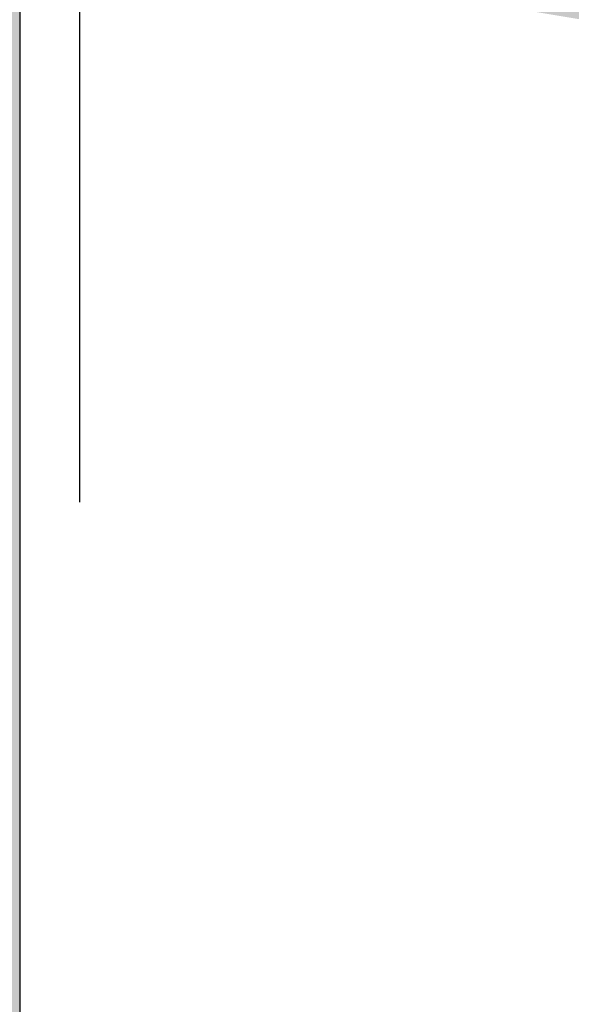
# Model space of a CAD drawing. Units: inches. Extents: x 2091 to 2899, y 967 to 2217.
# Tile 247 of 256: x 2212.144 to 2213.361, y 1137.765 to 1139.939. Entities that reach past the tile are written whole.
import ezdxf

# ---------------------------------------------------------------- set-up
doc = ezdxf.new("R2010")
doc.units = ezdxf.units.IN
doc.layers.add('A-ANNO-DIMS', color=2, linetype='Continuous', lineweight=18)
doc.layers.add('A-WALL-PATT', color=141, linetype='Continuous', lineweight=13, true_color=0xadddf7)
doc.styles.get("Standard").update_dxf_attribs({"font": 'arial.ttf'})
doc.dimstyles.new('ISO-25', dxfattribs={"dimtxt": 4, "dimasz": 4, "dimexe": 1.25, "dimexo": 0.625, "dimtad": 1, "dimdec": 0, "dimlunit": 3, "dimtxsty": 'Standard', "dimcen": 2.5, "dimadec": 0, "dimazin": 0, "dimtfac": 1, "dimtdec": 0, "dimtmove": 0, "dimatfit": 3, "dimfxl": 1, "dimarcsym": 0})

# ---------------------------------------------------------------- blocks, each defined once
blk = doc.blocks.new('*D37')
at = {"layer": 'A-ANNO-DIMS', "color": 0, "lineweight": -2, "transparency": 16777216}
for p, q in [((2203.1157, 1151.6221), (2203.1157, 1138.8736)), ((2212.2756, 1151.6221), (2212.2756, 1138.8736)), ((2199.1157, 1140.1236), (2195.1157, 1140.1236)), ((2203.1157, 1140.1236), (2212.2756, 1140.1236)), ((2216.2756, 1140.1236), (2245.9076, 1140.1236))]:
    blk.add_line(p, q, dxfattribs=at)
at = {"layer": 'A-ANNO-DIMS', "color": 0, "transparency": 16777216}
for points in [[(2199.1157, 1140.7902), (2199.1157, 1139.4569), (2203.1157, 1140.1236)], [(2216.2756, 1140.7902), (2216.2756, 1139.4569), (2212.2756, 1140.1236)]]:
    blk.add_solid(points, dxfattribs=at)
at = {"layer": 'Defpoints', "color": 0, "transparency": 16777216}
for p in [(2203.1157, 1152.2471), (2212.2756, 1152.2471), (2212.2756, 1140.1236)]:
    blk.add_point(p, dxfattribs=at)
at = {"layer": 'A-ANNO-DIMS', "color": 0, "transparency": 16777216, "insert": (2233.0916, 1142.7908), "char_height": 4, "attachment_point": 5}
blk.add_mtext('0\'-9" TYP.', dxfattribs=at)
blk = doc.blocks.new('*D71')
at = {"layer": 'A-ANNO-DIMS', "color": 0, "lineweight": -2, "transparency": 16777216}
for p, q in [((2212.1436, 1351.2941), (2212.1436, 969.4643)), ((2452.1436, 1351.2941), (2452.1436, 969.4643)), ((2216.1436, 970.7143), (2448.1436, 970.7143))]:
    blk.add_line(p, q, dxfattribs=at)
at = {"layer": 'A-ANNO-DIMS', "color": 0, "transparency": 16777216}
for points in [[(2216.1436, 971.381), (2216.1436, 970.0476), (2212.1436, 970.7143)], [(2448.1436, 971.381), (2448.1436, 970.0476), (2452.1436, 970.7143)]]:
    blk.add_solid(points, dxfattribs=at)
at = {"layer": 'Defpoints', "color": 0, "transparency": 16777216}
for p in [(2212.1436, 1351.9191), (2452.1436, 1351.9191), (2452.1436, 970.7143)]:
    blk.add_point(p, dxfattribs=at)
at = {"layer": 'A-ANNO-DIMS', "color": 0, "transparency": 16777216, "insert": (2332.1436, 973.3816), "char_height": 4, "attachment_point": 5}
blk.add_mtext('20\'-0"', dxfattribs=at)
blk = doc.blocks.new('*D75')
at = {"layer": 'A-ANNO-DIMS', "color": 0, "lineweight": -2, "transparency": 16777216}
for p, q in [((2212.1436, 1274.7941), (2212.1436, 969.4643)), ((2308.1436, 1274.7941), (2308.1436, 969.4643)), ((2216.1436, 970.7143), (2304.1436, 970.7143))]:
    blk.add_line(p, q, dxfattribs=at)
at = {"layer": 'A-ANNO-DIMS', "color": 0, "transparency": 16777216}
for points in [[(2216.1436, 971.381), (2216.1436, 970.0476), (2212.1436, 970.7143)], [(2304.1436, 971.381), (2304.1436, 970.0476), (2308.1436, 970.7143)]]:
    blk.add_solid(points, dxfattribs=at)
at = {"layer": 'Defpoints', "color": 0, "transparency": 16777216}
for p in [(2212.1436, 1275.4191), (2308.1436, 1275.4191), (2308.1436, 970.7143)]:
    blk.add_point(p, dxfattribs=at)
at = {"layer": 'A-ANNO-DIMS', "color": 0, "transparency": 16777216, "insert": (2260.1436, 973.3816), "char_height": 4, "attachment_point": 5}
blk.add_mtext('8\'-0"', dxfattribs=at)
blk = doc.blocks.new('*D91')
at = {"layer": 'A-ANNO-DIMS', "color": 0, "lineweight": -2, "transparency": 16777216}
for p, q in [((2211.6506, 1152.2471), (2098.3113, 1152.2471)), ((2099.5613, 1103.9191), (2099.5613, 1148.2471)), ((2211.5186, 1099.9191), (2098.3113, 1099.9191))]:
    blk.add_line(p, q, dxfattribs=at)
at = {"layer": 'A-ANNO-DIMS', "color": 0, "transparency": 16777216}
for points in [[(2098.8947, 1148.2471), (2100.228, 1148.2471), (2099.5613, 1152.2471)], [(2098.8947, 1103.9191), (2100.228, 1103.9191), (2099.5613, 1099.9191)]]:
    blk.add_solid(points, dxfattribs=at)
at = {"layer": 'Defpoints', "color": 0, "transparency": 16777216}
for p in [(2099.5613, 1152.2471), (2212.2756, 1152.2471), (2212.1436, 1099.9191)]:
    blk.add_point(p, dxfattribs=at)
at = {"layer": 'A-ANNO-DIMS', "color": 0, "transparency": 16777216, "insert": (2096.8681, 1126.0831), "char_height": 4, "attachment_point": 5, "rotation": 90}
blk.add_mtext('4\'-4 1/2"', dxfattribs=at)

msp = doc.modelspace()

# ---------------------------------------------------------------- hatches: boundary and pattern name
at = {"layer": 'A-WALL-PATT'}
h = msp.add_hatch(color=256, dxfattribs=at)
h.dxf.hatch_style = 1
h.paths.add_polyline_path([(2803.1436, 2050.9191), (2203.1436, 2050.9191), (2203.1436, 1090.9191), (2803.1436, 1090.9191)])
h.paths.add_polyline_path([(2635.7989, 1147.5405), (2674.5241, 1147.5405, 0.376086), (2678.5297, 1152.8802), (2678.5297, 1159.5565, 0.333335), (2674.5243, 1163.5618), (2674.5243, 1163.5619), (2674.5243, 1192.9344), (2635.806, 1192.9344), (2597.0876, 1192.9344), (2597.0876, 1163.5618, 0.333335), (2593.0823, 1159.5565), (2593.0823, 1152.8802, 0.376086), (2597.0879, 1147.5405)], flags=0)
h.paths.add_polyline_path([(2436.0104, 1278.2408, 0.000483), (2435.9526, 1278.215, -0.001328), (2435.9356, 1278.1117, -0.001711), (2436.1164, 1278.0408, 0.002185)], flags=0)
h.paths.add_polyline_path([(2794.1436, 1143.4191), (2794.1436, 1347.4191), (2543.3702, 1347.4191), (2543.3702, 1351.9191), (2794.1436, 1351.9191), (2794.1436, 1392.7136), (2793.9474, 1392.7136), (2793.9474, 1473.5369), (2794.1436, 1473.5369), (2794.1436, 1531.9191), (2650.1436, 1531.9191), (2650.1436, 1536.4191), (2794.1436, 1536.4191), (2794.1436, 1692.4191), (2609.3756, 1692.4191), (2609.3756, 1644.4191), (2604.8756, 1644.4191), (2604.8756, 1744.9191), (2609.3756, 1744.9191), (2609.3756, 1696.9191), (2794.1436, 1696.9191), (2794.1436, 1780.9191), (2609.6436, 1780.9191), (2493.8756, 1780.9191), (2493.8756, 1785.4191), (2609.6436, 1785.4191), (2794.1436, 1785.4191), (2794.1436, 1847.9388), (2793.9512, 1847.9388), (2793.9512, 1928.7622), (2794.1436, 1928.7622), (2794.1436, 1941.4191), (2614.1436, 1941.4191), (2614.1436, 1821.4191), (2609.6436, 1821.4191), (2609.6436, 1941.4191), (2392.1436, 1941.4191), (2392.1436, 1819.9191), (2387.6436, 1819.9191), (2387.6436, 1941.4191), (2212.1436, 1941.4191), (2212.1436, 1783.9191), (2392.1436, 1783.9191), (2392.1436, 1780.9191), (2212.1436, 1780.9191), (2212.1436, 1629.4191), (2387.6436, 1629.4191), (2387.6436, 1744.9191), (2392.1436, 1744.9191), (2392.1436, 1627.9191), (2317.1436, 1627.9191), (2317.1436, 1551.4191), (2317.1436, 1536.4191), (2459.3836, 1536.4191), (2459.3836, 1602.3965), (2463.8836, 1602.3965), (2463.8836, 1531.9191), (2456.6436, 1531.9191), (2456.6436, 1529.9191), (2452.1436, 1529.9191), (2452.1436, 1531.9191), (2312.6436, 1531.9191), (2312.6436, 1551.4191), (2306.1436, 1551.4191), (2306.1436, 1555.9191), (2308.1436, 1555.9191), (2308.1436, 1551.4191), (2312.6436, 1551.4191), (2312.6436, 1627.9191), (2212.1436, 1627.9191), (2212.1436, 1555.9191), (2270.1436, 1555.9191), (2270.1436, 1551.4191), (2212.1436, 1551.4191), (2212.1436, 1351.9191), (2272.1436, 1351.9191), (2272.1436, 1347.4191), (2212.1436, 1347.4191), (2212.1436, 1275.4191), (2308.1436, 1275.4191), (2308.1436, 1351.9191), (2452.1436, 1351.9191), (2452.1436, 1493.9191), (2456.6436, 1493.9191), (2456.6436, 1347.4191), (2312.6436, 1347.4191), (2312.6436, 1270.9191), (2212.1436, 1270.9191), (2212.1436, 1099.9191), (2281.2375, 1099.9191), (2282.871, 1110.9138), (2282.0083, 1116.9966), (2278.5577, 1121.4204), (2268.2056, 1128.0562), (2272.0876, 1128.0562), (2273.8129, 1131.927), (2279.4203, 1134.6919), (2285.0278, 1135.2449), (2287.6158, 1137.4568), (2288.0471, 1138.0098), (2289.3411, 1140.7747), (2291.0665, 1139.6687), (2292.3605, 1135.2449), (2295.3798, 1136.9038), (2296.2425, 1135.7979), (2297.1052, 1133.033), (2300.1246, 1138.0098), (2303.1439, 1138.0098), (2304.4379, 1135.7979), (2303.1439, 1133.586), (2306.5946, 1134.6919), (2307.8887, 1133.033), (2310.908, 1135.2449), (2313.9274, 1134.1389), (2315.6269, 1132.4271), (2308.32, 1117.5496), (2290.2038, 1109.8079), (2288.9098, 1103.1721), (2289.2723, 1099.9191), (2434.9182, 1099.9191), (2431.5932, 1124.7881), (2429.9302, 1169.5531), (2430.9272, 1240.5197), (2435.6589, 1238.1861), (2437.1352, 1196.5541), (2438.7982, 1143.9731), (2442.6782, 1111.9981), (2446.5582, 1099.9191), (2794.1436, 1099.9191), (2794.1436, 1138.9191), (2548.0324, 1138.9191), (2548.0324, 1143.4191), (2548.0324, 1148.8191), (2546.6685, 1148.0316), (2528.6857, 1179.1786, 0.256256), (2512.0324, 1148.8191), (2512.0324, 1143.4191), (2512.0324, 1138.9191), (2507.5324, 1138.9191), (2507.5324, 1143.4191), (2507.5324, 1148.8191, 0.256256), (2490.8792, 1179.1786), (2472.8964, 1148.0316), (2471.5324, 1148.8191), (2471.5324, 1143.4191), (2467.0324, 1143.4191), (2467.0324, 1269.9458, 0.039061), (2460.91, 1273.5801), (2467.0324, 1273.5801), (2467.0324, 1286.3254, 0.014511), (2465.2162, 1286.7619), (2467.0324, 1287.0526), (2467.0324, 1323.4191), (2471.5324, 1323.4191), (2471.5324, 1148.8191), (2489.5324, 1179.996), (2490.8964, 1179.2085), (2490.8792, 1179.1786, -0.256256), (2507.5324, 1148.8191), (2507.5324, 1143.4191), (2512.0324, 1143.4191), (2512.0324, 1148.8191, -0.256256), (2528.6857, 1179.1786), (2528.6685, 1179.2085), (2530.0324, 1179.996), (2548.0324, 1148.8191), (2548.0324, 1143.4191)], flags=16)
h.paths.add_polyline_path([(2607.7685, 1200.9451), (2607.7685, 1265.0306), (2597.0876, 1281.052), (2619.7846, 1281.052), (2627.7953, 1337.1269), (2635.7989, 1337.1269), (2643.8167, 1337.1269), (2651.8274, 1281.052), (2674.5243, 1281.052), (2663.8434, 1265.0306), (2663.8434, 1200.9451), (2635.806, 1200.9451)], flags=0)
edge = h.paths.add_edge_path(flags=0)
edge.add_ellipse((13303.8962, 1272.9987), major_axis=(-10595.313, 0), ratio=0.8423038701, start_angle=0.62823722, end_angle=0.6465541, ccw=False)
edge.add_ellipse((2711.7004, 1156.8527), major_axis=(2.2198, 0), ratio=0.842304, start_angle=111.5352, end_angle=180.6282, ccw=False)
edge.add_ellipse((13303.1563, 1272.9987), major_axis=(-10593.0263, 0), ratio=0.8423038695, start_angle=0.52827147, end_angle=0.6465541, ccw=False)
edge.add_line((2710.7646, 1175.3333), (2710.13, 1175.3333))
edge.add_ellipse((2710.13, 1176.5798), major_axis=(1.4798, 0), ratio=0.842304, start_angle=180, end_angle=270, ccw=False)
edge.add_line((2708.6501, 1176.5798), (2708.6501, 1200.7829))
edge.add_ellipse((2710.13, 1200.7829), major_axis=(1.4798, 0), ratio=0.842304, start_angle=90, end_angle=180, ccw=False)
edge.add_line((2710.13, 1202.0294), (2710.4651, 1202.0294))
edge.add_ellipse((13303.1563, 1272.9987), major_axis=(-10593.0263, 0), ratio=0.8423038695, start_angle=-0.09022909, end_angle=0.38386678, ccw=False)
edge.add_ellipse((2710.13, 1290.927), major_axis=(-1.4798, 0), ratio=0.842304, start_angle=0, end_angle=90, ccw=False)
edge.add_line((2708.6501, 1290.927), (2708.6501, 1315.1302))
edge.add_ellipse((2710.13, 1315.1302), major_axis=(-1.4798, 0), ratio=0.842304, start_angle=-90, end_angle=0, ccw=False)
edge.add_line((2710.13, 1316.3767), (2710.7063, 1316.3767))
edge.add_ellipse((3238.4017, 1296.2896), major_axis=(528.234, 0), ratio=0.84230387, start_angle=176.349572, end_angle=177.82005, ccw=False)
edge.add_ellipse((2775.063, 1071.4507), major_axis=(313.3078, 0), ratio=0.84230387, start_angle=102.125966, end_angle=103.780529, ccw=False)
edge.add_ellipse((2775.063, 1078.3057), major_axis=(-305.3029, 0), ratio=0.84230387, start_angle=-79.790461, end_angle=-77.555373, ccw=False)
edge.add_ellipse((2695.1418, 1541.9754), major_axis=(-250.9602, 0), ratio=0.84230387, start_angle=99.256566, end_angle=102.554933)
edge.add_line((2741.4103, 1334.2143), (2747.1325, 1337.3785))
edge.add_ellipse((2747.5386, 1336.8575), major_axis=(-0.7399, 0), ratio=0.842304, start_angle=270, end_angle=307.9331, ccw=False)
edge.add_ellipse((2747.5386, 1336.8575), major_axis=(-0.7399, 0), ratio=0.842304, start_angle=232.0669, end_angle=270, ccw=False)
edge.add_line((2747.9447, 1337.3785), (2753.6669, 1334.2143))
edge.add_ellipse((2799.9355, 1541.9754), major_axis=(250.9602, 0), ratio=0.84230387, start_angle=257.445067, end_angle=260.743434)
edge.add_ellipse((2720.0142, 1078.3057), major_axis=(305.3029, 0), ratio=0.84230387, start_angle=77.555373, end_angle=79.790461, ccw=False)
edge.add_ellipse((2720.0142, 1071.4507), major_axis=(-313.3078, 0), ratio=0.84230387, start_angle=256.219471, end_angle=257.874034, ccw=False)
edge.add_ellipse((2256.6755, 1296.2896), major_axis=(-528.234, 0), ratio=0.84230387, start_angle=182.17995, end_angle=183.650428, ccw=False)
edge.add_line((2784.3709, 1316.3767), (2784.9472, 1316.3767))
edge.add_ellipse((2784.9472, 1315.1302), major_axis=(1.4798, 0), ratio=0.842304, start_angle=0, end_angle=90, ccw=False)
edge.add_line((2786.4271, 1315.1302), (2786.4271, 1290.927))
edge.add_ellipse((2784.9472, 1290.927), major_axis=(1.4798, 0), ratio=0.842304, start_angle=270, end_angle=360, ccw=False)
edge.add_ellipse((-7808.0791, 1272.9987), major_axis=(10593.0263, 0), ratio=0.8423038695, start_angle=-0.38386678, end_angle=0.09022909, ccw=False)
edge.add_line((2784.6122, 1202.0294), (2784.9472, 1202.0294))
edge.add_ellipse((2784.9472, 1200.7829), major_axis=(1.4798, 0), ratio=0.842304, start_angle=0, end_angle=90, ccw=False)
edge.add_line((2786.4271, 1200.7829), (2786.4271, 1176.5798))
edge.add_ellipse((2784.9472, 1176.5798), major_axis=(-1.4798, 0), ratio=0.842304, start_angle=90, end_angle=180, ccw=False)
edge.add_line((2784.9472, 1175.3333), (2784.3126, 1175.3333))
edge.add_ellipse((-7808.0791, 1272.9987), major_axis=(10593.0263, 0), ratio=0.8423038695, start_angle=-0.6186432, end_angle=-0.52827147, ccw=False)
edge.add_ellipse((2783.3768, 1156.8527), major_axis=(-2.2198, 0), ratio=0.842304, start_angle=179.3718, end_angle=248.4648, ccw=False)
edge.add_ellipse((-7808.819, 1272.9987), major_axis=(-10595.313, 0), ratio=0.8423038658, start_angle=179.35344592, end_angle=179.3717628, ccw=False)
edge.add_ellipse((2780.2973, 1153.5008), major_axis=(-5.2464, 0), ratio=0.842304, start_angle=90, end_angle=179.3534, ccw=False)
edge.add_line((2780.2973, 1149.0817), (2714.7799, 1149.0817))
edge.add_ellipse((2714.7799, 1153.5008), major_axis=(5.2464, 0), ratio=0.842304, start_angle=180.6466, end_angle=270, ccw=False)
edge = h.paths.add_edge_path(flags=0)
edge.add_line((2718.1874, 1151.0078), (2718.1874, 1170.4724))
edge.add_ellipse((2721.1471, 1170.4724), major_axis=(-2.9597, 0), ratio=0.842304, start_angle=-90, end_angle=0, ccw=False)
edge.add_line((2721.1471, 1172.9653), (2773.9302, 1172.9653))
edge.add_ellipse((2773.9302, 1170.4724), major_axis=(-2.9597, 0), ratio=0.842304, start_angle=180, end_angle=270, ccw=False)
edge.add_line((2776.8899, 1170.4724), (2776.8899, 1151.0078))
edge.add_line((2776.8899, 1151.0078), (2718.1874, 1151.0078))
edge = h.paths.add_edge_path(flags=0)
edge.add_line((2718.1874, 1180.2342), (2718.1874, 1199.0578))
edge.add_ellipse((2747.5386, 1320.3986), major_axis=(147.0179, 0), ratio=0.84230387, start_angle=256.401865, end_angle=283.598135)
edge.add_line((2776.8899, 1199.0578), (2776.8899, 1180.2342))
edge.add_ellipse((2747.5386, 1301.575), major_axis=(147.0179, 0), ratio=0.84230387, start_angle=256.401865, end_angle=283.598135, ccw=False)
edge = h.paths.add_edge_path(flags=0)
edge.add_ellipse((13303.1563, 1272.9987), major_axis=(-10591.5465, 0), ratio=0.8423038696, start_angle=0.05559431, end_angle=0.37776419, ccw=False)
edge.add_line((2711.6169, 1262.7217), (2715.6674, 1249.4954))
edge.add_ellipse((6413.892, 1241.6919), major_axis=(-3698.2362, 0), ratio=0.84230387, start_angle=-0.1208974, end_angle=0.3640763)
edge.add_line((2715.761, 1218.1925), (2711.9343, 1203.1674))
edge = h.paths.add_edge_path(flags=0)
edge.add_line((2718.1874, 1251.0746), (2716.0025, 1267.4504))
edge.add_ellipse((2742.1512, 1202.1895), major_axis=(81.7726, 0), ratio=0.8423039, start_angle=94.277421, end_angle=111.834954, ccw=False)
edge.add_line((2737.0097, 1270.9306), (2758.0675, 1270.9306))
edge.add_ellipse((2752.9261, 1202.1895), major_axis=(81.7726, 0), ratio=0.8423039, start_angle=68.165046, end_angle=85.722579, ccw=False)
edge.add_line((2779.0747, 1267.4504), (2776.8899, 1251.0746))
edge.add_ellipse((2750.3381, 1187.8854), major_axis=(79.5797, 0), ratio=0.8423039, start_angle=67.208085, end_angle=85.12993)
edge.add_line((2756.0347, 1254.7437), (2739.0426, 1254.7437))
edge.add_ellipse((2744.7392, 1187.8854), major_axis=(79.5797, 0), ratio=0.8423039, start_angle=94.87007, end_angle=112.791915)
edge = h.paths.add_edge_path(flags=0)
edge.add_line((2783.1429, 1203.1674), (2779.3162, 1218.1925))
edge.add_ellipse((-918.8147, 1241.6919), major_axis=(3698.2362, 0), ratio=0.84230387, start_angle=-0.3640763, end_angle=0.1208974)
edge.add_line((2779.4098, 1249.4954), (2783.4604, 1262.7217))
edge.add_ellipse((-7808.0791, 1272.9987), major_axis=(-10591.5465, 0), ratio=0.8423038695, start_angle=179.62223581, end_angle=179.94440569, ccw=False)
edge = h.paths.add_edge_path(flags=0)
edge.add_ellipse((2734.2009, 1286.6904), major_axis=(-0.3566, 6.3401), ratio=0.603834, start_angle=89.00201, end_angle=253.65741, ccw=False)
edge.add_line((2730.369, 1286.5418), (2730.369, 1301.352))
edge.add_line((2730.369, 1301.352), (2735.9133, 1305.2148))
edge.add_ellipse((2736.3849, 1304.7346), major_axis=(0.7399, 0), ratio=0.842304, start_angle=90, end_angle=134.4802, ccw=False)
edge.add_line((2736.3849, 1305.3578), (2738.0328, 1305.3578))
edge.add_line((2738.0328, 1305.3578), (2738.0328, 1307.7079))
edge.add_ellipse((2794.2016, 1307.7079), major_axis=(56.1689, 0), ratio=0.8423039, start_angle=150.56143, end_angle=180, ccw=False)
edge.add_ellipse((2700.8756, 1307.7079), major_axis=(-56.1689, 0), ratio=0.8423039, start_angle=180, end_angle=209.43857, ccw=False)
edge.add_line((2757.0444, 1307.7079), (2757.0444, 1305.3578))
edge.add_line((2757.0444, 1305.3578), (2758.6923, 1305.3578))
edge.add_ellipse((2758.6923, 1304.7346), major_axis=(-0.7399, 0), ratio=0.842304, start_angle=225.5198, end_angle=270, ccw=False)
edge.add_line((2759.1639, 1305.2148), (2764.7082, 1301.352))
edge.add_line((2764.7082, 1301.352), (2764.7082, 1286.5418))
edge.add_ellipse((2760.8763, 1286.6904), major_axis=(0.3566, 6.3401), ratio=0.603834, start_angle=106.34259, end_angle=270.99799, ccw=False)
edge.add_line((2757.0444, 1285.7971), (2757.0444, 1307.7079))
edge.add_ellipse((2700.8756, 1307.7079), major_axis=(-56.1689, 0), ratio=0.8423039, start_angle=180, end_angle=209.43857)
edge.add_ellipse((2794.2016, 1307.7079), major_axis=(56.1689, 0), ratio=0.8423039, start_angle=150.56143, end_angle=180)
edge.add_line((2738.0328, 1307.7079), (2738.0328, 1285.7971))
h.paths.add_polyline_path([(2417.8123, 1104.4497), (2413.4923, 1102.5297), (2410.6123, 1103.9697), (2409.1723, 1106.3697), (2407.2523, 1107.3297), (2406.2923, 1109.7297), (2405.3323, 1114.0497), (2405.3323, 1117.8897), (2406.2923, 1120.1297), (2407.2523, 1119.8097), (2408.8483, 1118.3277), (2410.1739, 1119.4242), (2410.2113, 1120.4057), (2411.0407, 1121.4191), (2410.6993, 1119.8587), (2410.1739, 1119.4242), (2410.0885, 1117.1761), (2411.1328, 1116.2063), (2413.9723, 1119.3297), (2416.8523, 1120.7697), (2416.8697, 1120.7988), (2417.0351, 1119.4051), (2417.8962, 1118.1434), (2418.2923, 1118.3697), (2419.5444, 1120.0393), (2419.3609, 1118.3875), (2419.0321, 1119.3562), (2418.3989, 1118.5119), (2419.2523, 1114.5297), (2418.7941, 1107.1988)], flags=0)
h.paths.add_polyline_path([(2508.8702, 1347.4191), (2508.3702, 1347.4191), (2508.3702, 1351.9191), (2508.8702, 1351.9191)], flags=0)
h.paths.add_polyline_path([(2473.3702, 1347.4191), (2472.3702, 1347.4191), (2467.8702, 1347.4191), (2467.8702, 1455.4191), (2472.3702, 1455.4191), (2472.3702, 1352.4191), (2473.3702, 1352.4191)], flags=0)
h.paths.add_polyline_path([(2352.1062, 1217.4462), (2349.2262, 1218.8862), (2347.7862, 1221.2862), (2345.8662, 1222.2462), (2344.9062, 1224.6462), (2343.9462, 1228.9662), (2343.9462, 1232.8062), (2344.9062, 1235.0462), (2345.8662, 1234.7262), (2347.4623, 1233.2442), (2348.7879, 1234.3407), (2348.8252, 1235.3222), (2349.6547, 1236.3355), (2349.3132, 1234.7752), (2348.7879, 1234.3407), (2348.7024, 1232.0926), (2349.7468, 1231.1228), (2352.5862, 1234.2462), (2355.4662, 1235.6862), (2355.4837, 1235.7153), (2355.649, 1234.3216), (2356.5102, 1233.0599), (2356.9062, 1233.2862), (2358.1584, 1234.9558), (2357.9749, 1233.304), (2357.6461, 1234.2726), (2357.0129, 1233.4284), (2357.8662, 1229.4462), (2357.4081, 1222.1153), (2356.4262, 1219.3662)], flags=0)
h.paths.add_polyline_path([(2348.2968, 1112.2244), (2347.0138, 1112.3104), (2345.5298, 1114.1274), (2345.7318, 1115.8584), (2346.8118, 1116.9824), (2346.8118, 1114.6464), (2345.8668, 1114.2144), (2346.8798, 1114.3004)], flags=0)
h.paths.add_polyline_path([(2347.0138, 1110.9264), (2346.2718, 1110.4934), (2346.6098, 1111.1864)], flags=0)
h.paths.add_polyline_path([(2345.8668, 1118.1944), (2345.5298, 1117.3294), (2343.7078, 1118.0214), (2344.3828, 1118.6264)], flags=0)
h.paths.add_polyline_path([(2346.6768, 1109.2824), (2346.0698, 1108.0714), (2345.8668, 1110.0614)], flags=0)
h.paths.add_polyline_path([(2345.0568, 1119.7514), (2343.6398, 1119.7514), (2343.9778, 1121.1354)], flags=0)
h.paths.add_polyline_path([(2345.2598, 1116.5504), (2345.1248, 1115.8584), (2344.9218, 1115.6854), (2344.7198, 1116.3774)], flags=0)
h.paths.add_polyline_path([(2345.6648, 1112.3104), (2345.4618, 1111.5324), (2344.0448, 1111.9644), (2344.6518, 1112.5704)], flags=0)
h.paths.add_polyline_path([(2345.1918, 1113.3494), (2344.4498, 1113.8684), (2344.7198, 1114.3874)], flags=0)
h.paths.add_polyline_path([(2344.6518, 1116.8094), (2344.1798, 1115.6854), (2344.6518, 1115.3394), (2343.9098, 1114.9064), (2343.0328, 1115.9444), (2343.6398, 1116.4634)], flags=0)
h.paths.add_polyline_path([(2345.8668, 1106.6864), (2344.9898, 1105.5624), (2344.5168, 1106.6004)], flags=0)
h.paths.add_polyline_path([(2344.8548, 1110.0614), (2344.5168, 1109.2824), (2344.1128, 1109.7154)], flags=0)
h.paths.add_polyline_path([(2344.0448, 1113.5224), (2343.4378, 1113.0894), (2342.7628, 1113.9544)], flags=0)
h.paths.add_polyline_path([(2344.3148, 1111.0124), (2342.9648, 1110.3204), (2342.9648, 1111.0994)], flags=0)
h.paths.add_polyline_path([(2345.1248, 1104.6974), (2344.5848, 1103.7454), (2344.4498, 1104.2644)], flags=0)
h.paths.add_polyline_path([(2342.8298, 1121.2224), (2341.7498, 1120.5304), (2340.5358, 1121.0494), (2340.1308, 1121.8284), (2340.6708, 1122.9524), (2341.1428, 1121.8284), (2341.6148, 1122.0014)], flags=0)
h.paths.add_polyline_path([(2342.9648, 1119.7514), (2343.0328, 1118.4534), (2342.0878, 1118.0214), (2342.0198, 1119.4914)], flags=0)
h.paths.add_polyline_path([(2342.6948, 1116.8964), (2341.9528, 1116.6364), (2342.0198, 1117.3294)], flags=0)
h.paths.add_polyline_path([(2343.0328, 1112.2244), (2342.0198, 1111.7914), (2341.5478, 1112.2244), (2342.3578, 1113.3494)], flags=0)
h.paths.add_polyline_path([(2343.7748, 1104.4374), (2342.6278, 1102.8804), (2342.6948, 1104.6104), (2343.4378, 1105.1294)], flags=0)
h.paths.add_polyline_path([(2342.0198, 1115.0794), (2340.8058, 1115.5124), (2340.9408, 1116.3774)], flags=0)
h.paths.add_polyline_path([(2341.4808, 1120.0974), (2341.4808, 1119.4054), (2341.0758, 1119.5784), (2341.1428, 1120.0974)], flags=0)
h.paths.add_polyline_path([(2341.8178, 1114.4734), (2340.9408, 1113.0894), (2340.8058, 1114.5604)], flags=0)
h.paths.add_polyline_path([(2341.1428, 1118.5404), (2340.9408, 1116.9824), (2339.0508, 1117.6754), (2339.0508, 1118.6264)], flags=0)
h.paths.add_polyline_path([(2342.6948, 1101.6684), (2341.9528, 1101.8414), (2342.5598, 1102.3614)], flags=0)
h.paths.add_polyline_path([(2340.3328, 1119.6654), (2338.4438, 1119.5784), (2337.9038, 1120.3574), (2339.6578, 1120.6164)], flags=0)
h.paths.add_polyline_path([(2340.3328, 1115.3394), (2340.0628, 1113.6954), (2339.3878, 1115.3394)], flags=0)
h.paths.add_polyline_path([(2341.8178, 1103.8314), (2341.5478, 1102.8804), (2341.1428, 1103.6584)], flags=0)
h.paths.add_polyline_path([(2339.0508, 1122.8664), (2337.2958, 1121.8284), (2337.0938, 1123.1254), (2337.7688, 1123.8184)], flags=0)
h.paths.add_polyline_path([(2339.1178, 1121.7414), (2338.8478, 1121.2224), (2338.1738, 1121.0494), (2338.3758, 1121.5684)], flags=0)
h.paths.add_polyline_path([(2339.1858, 1119.3194), (2338.6458, 1118.7134), (2338.2408, 1118.1074), (2338.2408, 1118.8864)], flags=0)
h.paths.add_polyline_path([(2341.1428, 1101.9284), (2340.6028, 1101.2364), (2340.0628, 1101.8414), (2340.6028, 1102.3614)], flags=0)
h.paths.add_polyline_path([(2337.6338, 1117.7614), (2336.6208, 1118.2804), (2337.2958, 1118.9724)], flags=0)
h.paths.add_polyline_path([(2336.8238, 1119.5784), (2334.7988, 1118.9724), (2335.2038, 1120.3574), (2336.5538, 1120.8764)], flags=0)
h.paths.add_polyline_path([(2339.1178, 1100.4574), (2337.3638, 1100.5434), (2336.7558, 1101.2364)], flags=0)
h.paths.add_polyline_path([(2336.3508, 1122.4334), (2336.0138, 1121.9144), (2334.9338, 1122.4334), (2334.5288, 1123.4714), (2335.7438, 1122.7794)], flags=0)
h.paths.add_polyline_path([(2334.7318, 1120.8764), (2334.2588, 1120.3574), (2334.0568, 1120.7894), (2334.5968, 1121.3084)], flags=0)
h.paths.add_polyline_path([(2334.4618, 1122.1744), (2332.5718, 1121.3084), (2331.3568, 1122.1744), (2332.0998, 1122.8664)], flags=0)
h.paths.add_polyline_path([(2334.2588, 1118.5404), (2333.3818, 1118.4534), (2333.6518, 1119.3194)], flags=0)
h.paths.add_polyline_path([(2335.5418, 1102.2744), (2334.1918, 1102.6204), (2335.2718, 1103.3124)], flags=0)
h.paths.add_polyline_path([(2332.7068, 1119.6654), (2331.6948, 1120.4434), (2332.5048, 1120.7894)], flags=0)
h.paths.add_polyline_path([(2334.7318, 1101.1494), (2333.5168, 1101.5824), (2333.9888, 1101.7554)], flags=0)
h.paths.add_polyline_path([(2332.6398, 1116.6364), (2331.0868, 1116.2904), (2331.9648, 1118.1944)], flags=0)
h.paths.add_polyline_path([(2330.7498, 1121.5684), (2330.2768, 1120.2704), (2328.5228, 1119.3194), (2328.9948, 1121.0494)], flags=0)
h.paths.add_polyline_path([(2330.7498, 1118.6264), (2330.0078, 1117.5024), (2329.8728, 1118.0214)], flags=0)
h.paths.add_polyline_path([(2332.0998, 1102.3614), (2330.5468, 1102.0144), (2331.6948, 1102.9664)], flags=0)
h.paths.add_polyline_path([(2329.5348, 1113.6084), (2329.0628, 1112.3104), (2328.5898, 1113.3494)], flags=0)
h.paths.add_polyline_path([(2328.3878, 1117.8484), (2327.5098, 1116.5504), (2327.1728, 1117.7614)], flags=0)
h.paths.add_polyline_path([(2329.7378, 1106.5134), (2329.5348, 1105.3024), (2328.2528, 1106.0814)], flags=0)
h.paths.add_polyline_path([(2328.6578, 1114.3874), (2328.0498, 1114.1274), (2328.3198, 1114.9064)], flags=0)
h.paths.add_polyline_path([(2328.3198, 1112.2244), (2327.1058, 1112.1374), (2326.7008, 1112.6564)], flags=0)
h.paths.add_polyline_path([(2326.9028, 1115.2524), (2326.7008, 1114.1274), (2325.2158, 1113.6084), (2326.0928, 1115.3394)], flags=0)
h.paths.add_polyline_path([(2326.6328, 1108.3304), (2326.0928, 1107.3794), (2325.8908, 1108.5034), (2326.4978, 1109.1094)], flags=0)
h.paths.add_polyline_path([(2615.1436, 1531.9191), (2609.6436, 1531.9191), (2609.6436, 1620.4191), (2614.1436, 1620.4191), (2614.1436, 1536.4191), (2615.1436, 1536.4191)], flags=0)
h.paths.add_polyline_path([(2545.1436, 1563.4191), (2464.1436, 1563.4191), (2464.1436, 1632.4191), (2509.1436, 1632.4191), (2509.1436, 1627.9191), (2509.1436, 1603.9191), (2468.6436, 1603.9191), (2468.6436, 1567.9191), (2540.6436, 1567.9191), (2540.6436, 1591.9191), (2545.1436, 1591.9191)], flags=0)
h.paths.add_polyline_path([(2388.969, 1549.9857), (2357.4342, 1549.9857), (2357.4342, 1623.3608), (2399.3628, 1623.3608), (2435.6895, 1623.3608), (2435.5925, 1602.5593), (2435.5925, 1602.3965), (2388.969, 1602.3965)], flags=0)
h.paths.add_polyline_path([(2388.8806, 1555.8092), (2374.9044, 1555.8092), (2374.9044, 1600.5716), (2374.9044, 1615.4576), (2406.3509, 1615.4576), (2406.3509, 1618.9394), (2412.1743, 1615.4576), (2406.3509, 1611.9759), (2406.3509, 1615.4576), (2388.8806, 1615.4576)], flags=0)
h.paths.add_polyline_path([(2568.8756, 1644.4191), (2453.3756, 1644.4191), (2453.3756, 1785.4191), (2457.8756, 1785.4191), (2457.8756, 1648.9191), (2568.8756, 1648.9191)], flags=0)
h.paths.add_polyline_path([(2212.1436, 1945.9191), (2212.1436, 2041.9191), (2794.1436, 2041.9191), (2794.1436, 1945.9191)], flags=16)
h.paths.add_polyline_path([(2271.0827, 1964.3172), (2776.853, 1964.3172), (2776.853, 2037.1696), (2271.0827, 2037.1696)], flags=8)
h.paths.add_polyline_path([(2380.6493, 1536.8241), (2461.0408, 1536.8241), (2461.0408, 1554.6526), (2380.6493, 1554.6526)], flags=8)
h.paths.add_polyline_path([(2240.7557, 1609.7255), (2309.1858, 1609.7255), (2309.1858, 1617.6982), (2240.7557, 1617.6982)], flags=8)
h.paths.add_polyline_path([(2212.6773, 1313.5041), (2282.5915, 1313.5041), (2282.5915, 1322.7452), (2212.6773, 1322.7452)], flags=8)
h.paths.add_polyline_path([(2457.112, 1114.7786), (2558.4816, 1114.7786), (2558.4816, 1142.2197), (2457.112, 1142.2197)], flags=8)
h.paths.add_polyline_path([(2473.4423, 1273.0101), (2604.6412, 1273.0101), (2604.6412, 1318.3469), (2473.4423, 1318.3469)], flags=8)
h.paths.add_polyline_path([(2638.8763, 1626.9774), (2684.2504, 1627.9767), (2684.0385, 1637.5975), (2638.6644, 1636.5982)], flags=8)
h.paths.add_polyline_path([(2537.5906, 1453.7934), (2628.3895, 1453.7934), (2628.3895, 1475.3448), (2537.5906, 1475.3448)], flags=8)
h.paths.add_polyline_path([(2504.1376, 1714.6324), (2554.6472, 1714.6324), (2554.6472, 1730.2377), (2504.1376, 1730.2377)], flags=8)
h.paths.add_polyline_path([(2487.5012, 1575.6519), (2535.0971, 1575.6519), (2535.0971, 1598.3776), (2487.5012, 1598.3776)], flags=8)
h.paths.add_polyline_path([(2709.0994, 1735.7103), (2740.0166, 1735.7103), (2740.0166, 1749.9376), (2709.0994, 1749.9376)], flags=8)
h.paths.add_polyline_path([(2442.4384, 1792.1717), (2564.7288, 1792.1717), (2564.7288, 1842.0002), (2442.4384, 1842.0002)], flags=8)
h.paths.add_polyline_path([(2655.8158, 1809.6441), (2789.5201, 1806.6938), (2790.085, 1832.2916), (2656.3806, 1835.2419)], flags=8)
h.paths.add_polyline_path([(2234.8427, 1797.7201), (2368.5929, 1794.7689), (2369.1607, 1820.5041), (2235.4106, 1823.4554)], flags=8)
h.paths.add_polyline_path([(2245.1385, 1644.0063), (2398.4277, 1640.6239), (2398.9948, 1666.3248), (2245.7056, 1669.7073)], flags=8)
h.paths.add_polyline_path([(2306.1428, 1431.1685), (2413.7683, 1428.7937), (2414.3331, 1454.3915), (2306.7077, 1456.7664)], flags=8)
h.paths.add_polyline_path([(2306.8346, 1458.2331), (2393.3805, 1456.3234), (2393.9328, 1481.3544), (2307.3869, 1483.2641)], flags=8)

# ---------------------------------------------------------------- dimensions: what is measured, and where the dimension line sits
at = {"layer": 'A-ANNO-DIMS'}
for base, p1, p2, picture, middle in [((2452.1436, 970.7143), (2212.1436, 1351.9191), (2452.1436, 1351.9191), '*D71', (2332.1436, 973.3816)), ((2308.1436, 970.7143), (2212.1436, 1275.4191), (2308.1436, 1275.4191), '*D75', (2260.1436, 973.3816))]:
    dim = msp.add_linear_dim(base=base, p1=p1, p2=p2, dimstyle='ISO-25', override={"dimdec": 1, "dimlfac": 1, "dimrnd": 0, "dimzin": 1, "dimdsep": 46, "dimlunit": 4, "dimfrac": 2}, dxfattribs=at)
    dim.commit()
    dim.dimension.update_dxf_attribs({"geometry": picture, "text_midpoint": middle})
dim = msp.add_linear_dim(base=(2099.5613, 1152.2471), p1=(2212.1436, 1099.9191), p2=(2212.2756, 1152.2471), angle=90, dimstyle='ISO-25', override={"dimdec": 1, "dimlfac": 1, "dimrnd": 0, "dimzin": 1, "dimdsep": 46, "dimlunit": 4, "dimfrac": 2}, dxfattribs=at)
dim.commit()
dim.dimension.update_dxf_attribs({"geometry": '*D91', "text_midpoint": (2096.8681, 1126.0831)})
dim = msp.add_linear_dim(base=(2212.2756, 1140.1236), p1=(2203.1157, 1152.2471), p2=(2212.2756, 1152.2471), text='<> TYP.', dimstyle='ISO-25', override={"dimdec": 1, "dimlfac": 1, "dimrnd": 0, "dimzin": 1, "dimdsep": 46, "dimlunit": 4, "dimfrac": 2}, dxfattribs=at)
dim.commit()
dim.dimension.update_dxf_attribs({"geometry": '*D37', "text_midpoint": (2233.0916, 1142.7908)})

doc.saveas('drawing.dxf')
